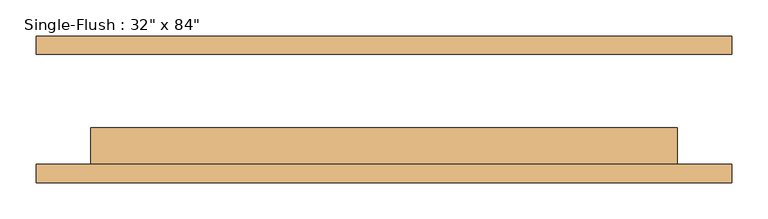
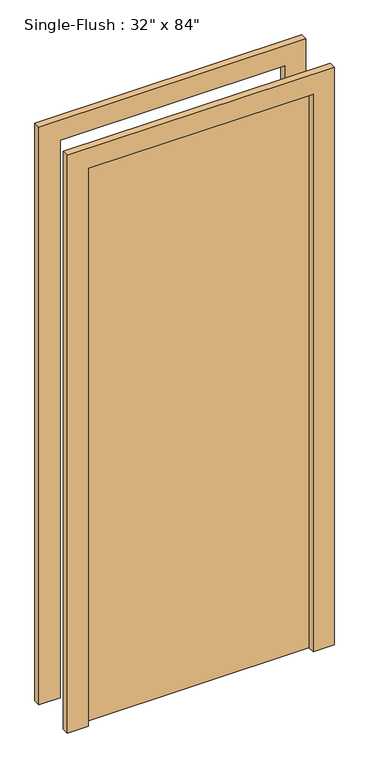
"""IFC4 building model written with IfcOpenShell, lengths in millimetres: door geometry."""

from ifc_helpers import new_model, si_unit, frame, origin, origin_with_axes, place, context, project, spatial, polyline, outline, extrude, source, transform, mapped, element, save


def door_bb092f7c(model_context):
    return source(origin(), model_context, "Body", "SweptSolid", [
        extrude(outline(polyline([(2209.8, -482.6), (0.0, -482.6), (0.0, -406.4), (2133.6, -406.4), (2133.6, 406.4), (0.0, 406.4), (0.0, 482.6), (2209.8, 482.6), (2209.8, -482.6)])), frame((0.0, -101.6, 0.0), z_axis=(0.0, 1.0, 0.0), x_axis=(0.0, 0.0, 1.0)), (0.0, 0.0, 1.0), 25.4),
        extrude(outline(polyline([(2209.8, 482.6), (2209.8, -482.6), (0.0, -482.6), (0.0, -406.4), (2133.6, -406.4), (2133.6, 406.4), (0.0, 406.4), (0.0, 482.6), (2209.8, 482.6)])), frame((0.0, 76.2, 0.0), z_axis=(0.0, 1.0, 0.0), x_axis=(0.0, 0.0, 1.0)), (0.0, 0.0, 1.0), 25.4),
        extrude(outline(polyline([(406.4, -25.4), (406.4, -76.2), (-406.4, -76.2), (-406.4, -25.4), (406.4, -25.4)])), origin_with_axes(), (0.0, 0.0, 1.0), 2133.6),
    ])


if __name__ == "__main__":
    model = new_model("IFC4")
    model_context = context("Model", 3, world=origin())
    ifc_project = project(units=[si_unit("LENGTHUNIT", "METRE", prefix="MILLI")], contexts=[model_context])
    site = spatial("IfcSite", under=ifc_project)
    building = spatial("IfcBuilding", under=site)
    placement = place(None, origin())
    door_shape = door_bb092f7c(model_context)
    element("IfcDoor", 1, ObjectType="Single-Flush : 32\" x 84\"", at=placement, inside=building, context=model_context, shape_type="MappedRepresentation", body=[
        mapped(door_shape, transform((0.0, 0.0, 0.0), x_axis=(1.0, 0.0, 0.0), y_axis=(0.0, 1.0, 0.0), z_axis=(0.0, 0.0, 1.0))),
    ])
    save(model, "model.ifc")

# Revit data of these elements
# Type "Single-Flush : 32\" x 84\""
#   Type Mark = "3"
#   Construction Type Id = "MDOOR"
#   Assembly Code = "C1020"
#   Analytic Construction = "Metal"
#   Thickness = 0' - 2"
#   Heat Transfer Coefficient (U) = 0.651978 BTU/(h·ft²·°F)
#   Height = 7' - 0"
#   Trim Projection Ext = 0' - 1"
#   Trim Projection Int = 0' - 1"
#   Trim Width = 0' - 3"
#   Width = 2' - 8"
#   Define Thermal Properties by = 1
#   Define Thermal Properties by = 1
#   Door Material = Door - Panel
#   Frame Material = Door - Frame
#   Visual Light Transmittance = 0
#   Solar Heat Gain Coefficient = 0
#   Function = (empty or 0)
#   Wall Closure = (empty or 0)
# Element 1 (IfcDoor, "Single-Flush : 32\" x 84\"")
#   Materials on its faces: "Door - Frame", "Door - Panel"
# Materials
#   "Door - Panel": class "Wood", colour RGB 210 159 95, transparency 0, Cost = 0
#   "Door - Frame": colour RGB 118 70 51, transparency 0, Cost = 0
